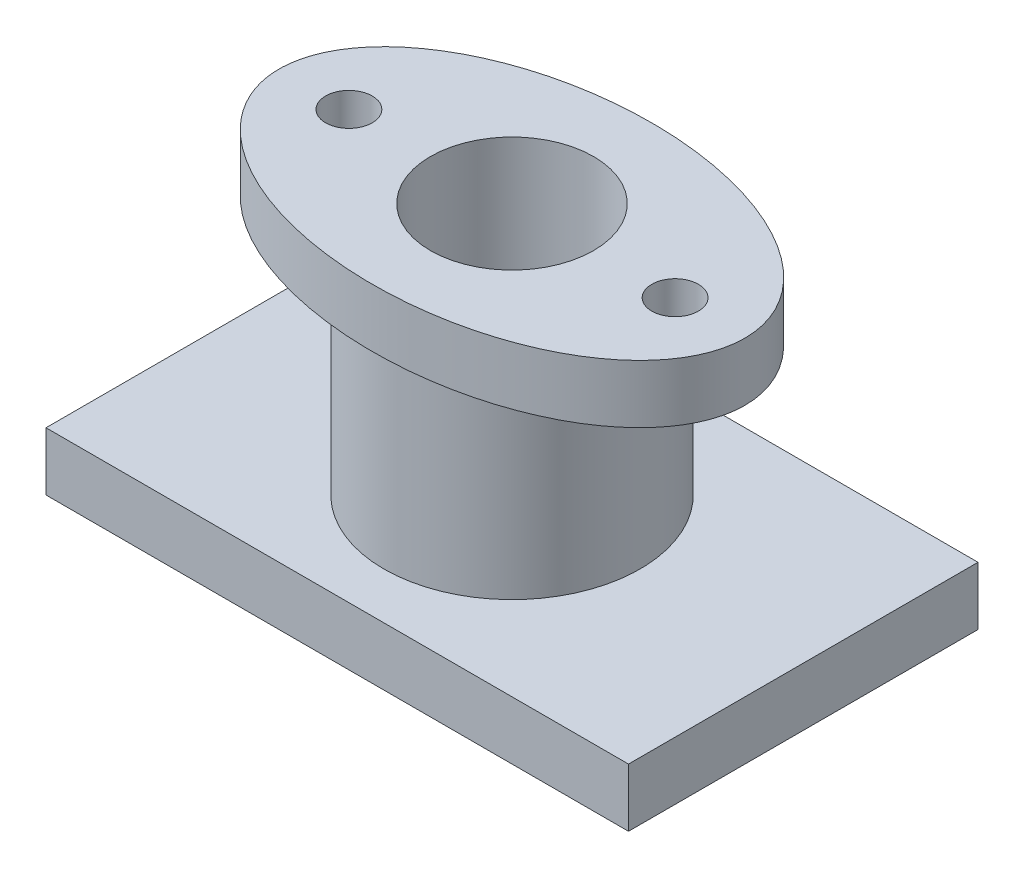
ISO-10303-21;
HEADER;
FILE_DESCRIPTION(('STEP AP214'),'2;1');
FILE_NAME('part.step','',(''),(''),'','','');
FILE_SCHEMA(('AUTOMOTIVE_DESIGN { 1 0 10303 214 1 1 1 1 }'));
ENDSEC;
DATA;
#1=APPLICATION_CONTEXT('core data for automotive mechanical design processes');
#2=APPLICATION_PROTOCOL_DEFINITION('international standard','automotive_design',2000,#1);
#3=PRODUCT_CONTEXT('',#1,'mechanical');
#4=PRODUCT('Part','Part','',(#3));
#5=PRODUCT_RELATED_PRODUCT_CATEGORY('part','',(#4));
#6=PRODUCT_DEFINITION_FORMATION('','',#4);
#7=PRODUCT_DEFINITION_CONTEXT('part definition',#1,'design');
#8=PRODUCT_DEFINITION('design','',#6,#7);
#9=PRODUCT_DEFINITION_SHAPE('','',#8);
#10=(LENGTH_UNIT() NAMED_UNIT(*) SI_UNIT(.MILLI.,.METRE.));
#11=(NAMED_UNIT(*) PLANE_ANGLE_UNIT() SI_UNIT($,.RADIAN.));
#12=(NAMED_UNIT(*) SI_UNIT($,.STERADIAN.) SOLID_ANGLE_UNIT());
#13=UNCERTAINTY_MEASURE_WITH_UNIT(LENGTH_MEASURE(1.E-05),#10,'distance_accuracy_value','');
#14=(GEOMETRIC_REPRESENTATION_CONTEXT(3) GLOBAL_UNCERTAINTY_ASSIGNED_CONTEXT((#13)) GLOBAL_UNIT_ASSIGNED_CONTEXT((#10,
#11,#12)) REPRESENTATION_CONTEXT('',''));
#15=CARTESIAN_POINT('',(0.,0.,0.));
#16=DIRECTION('',(0.,0.,1.));
#17=DIRECTION('',(1.,0.,0.));
#18=AXIS2_PLACEMENT_3D('',#15,#16,#17);
#19=CARTESIAN_POINT('',(75.,15.,45.));
#20=DIRECTION('',(-1.,0.,0.));
#21=DIRECTION('',(0.,0.,1.));
#22=AXIS2_PLACEMENT_3D('',#19,#20,#21);
#23=PLANE('',#22);
#24=DIRECTION('',(0.,0.,-1.));
#25=VECTOR('',#24,1.);
#26=CARTESIAN_POINT('',(75.,0.,45.));
#27=LINE('',#26,#25);
#28=CARTESIAN_POINT('',(75.,0.,45.));
#29=VERTEX_POINT('',#28);
#30=CARTESIAN_POINT('',(75.,0.,-45.));
#31=VERTEX_POINT('',#30);
#32=EDGE_CURVE('E102',#29,#31,#27,.T.);
#33=ORIENTED_EDGE('',*,*,#32,.T.);
#34=DIRECTION('',(0.,-1.,0.));
#35=VECTOR('',#34,1.);
#36=CARTESIAN_POINT('',(75.,15.,-45.));
#37=LINE('',#36,#35);
#38=CARTESIAN_POINT('',(75.,15.,-45.));
#39=VERTEX_POINT('',#38);
#40=EDGE_CURVE('E50',#39,#31,#37,.T.);
#41=ORIENTED_EDGE('',*,*,#40,.F.);
#42=DIRECTION('',(0.,0.,-1.));
#43=VECTOR('',#42,1.);
#44=CARTESIAN_POINT('',(75.,15.,45.));
#45=LINE('',#44,#43);
#46=CARTESIAN_POINT('',(75.,15.,45.));
#47=VERTEX_POINT('',#46);
#48=EDGE_CURVE('E91',#47,#39,#45,.T.);
#49=ORIENTED_EDGE('',*,*,#48,.F.);
#50=DIRECTION('',(0.,-1.,0.));
#51=VECTOR('',#50,1.);
#52=CARTESIAN_POINT('',(75.,15.,45.));
#53=LINE('',#52,#51);
#54=EDGE_CURVE('E103',#47,#29,#53,.T.);
#55=ORIENTED_EDGE('',*,*,#54,.T.);
#56=EDGE_LOOP('',(#33,#41,#49,#55));
#57=FACE_BOUND('',#56,.T.);
#58=ADVANCED_FACE('F39',(#57),#23,.F.);
#59=CARTESIAN_POINT('',(-75.,15.,-45.));
#60=DIRECTION('',(0.,0.,1.));
#61=DIRECTION('',(1.,0.,0.));
#62=AXIS2_PLACEMENT_3D('',#59,#60,#61);
#63=PLANE('',#62);
#64=DIRECTION('',(-1.,0.,0.));
#65=VECTOR('',#64,1.);
#66=CARTESIAN_POINT('',(-75.,0.,-45.));
#67=LINE('',#66,#65);
#68=CARTESIAN_POINT('',(-75.,0.,-45.));
#69=VERTEX_POINT('',#68);
#70=EDGE_CURVE('E98',#31,#69,#67,.T.);
#71=ORIENTED_EDGE('',*,*,#70,.T.);
#72=DIRECTION('',(0.,-1.,0.));
#73=VECTOR('',#72,1.);
#74=CARTESIAN_POINT('',(-75.,15.,-45.));
#75=LINE('',#74,#73);
#76=CARTESIAN_POINT('',(-75.,15.,-45.));
#77=VERTEX_POINT('',#76);
#78=EDGE_CURVE('E93',#77,#69,#75,.T.);
#79=ORIENTED_EDGE('',*,*,#78,.F.);
#80=DIRECTION('',(-1.,0.,0.));
#81=VECTOR('',#80,1.);
#82=CARTESIAN_POINT('',(-75.,15.,-45.));
#83=LINE('',#82,#81);
#84=EDGE_CURVE('E86',#39,#77,#83,.T.);
#85=ORIENTED_EDGE('',*,*,#84,.F.);
#86=ORIENTED_EDGE('',*,*,#40,.T.);
#87=EDGE_LOOP('',(#71,#79,#85,#86));
#88=FACE_BOUND('',#87,.T.);
#89=ADVANCED_FACE('F94',(#88),#63,.F.);
#90=CARTESIAN_POINT('',(-75.,15.,45.));
#91=DIRECTION('',(1.,0.,0.));
#92=DIRECTION('',(0.,0.,-1.));
#93=AXIS2_PLACEMENT_3D('',#90,#91,#92);
#94=PLANE('',#93);
#95=DIRECTION('',(0.,0.,1.));
#96=VECTOR('',#95,1.);
#97=CARTESIAN_POINT('',(-75.,0.,45.));
#98=LINE('',#97,#96);
#99=CARTESIAN_POINT('',(-75.,0.,45.));
#100=VERTEX_POINT('',#99);
#101=EDGE_CURVE('E75',#69,#100,#98,.T.);
#102=ORIENTED_EDGE('',*,*,#101,.T.);
#103=DIRECTION('',(0.,-1.,0.));
#104=VECTOR('',#103,1.);
#105=CARTESIAN_POINT('',(-75.,15.,45.));
#106=LINE('',#105,#104);
#107=CARTESIAN_POINT('',(-75.,15.,45.));
#108=VERTEX_POINT('',#107);
#109=EDGE_CURVE('E97',#108,#100,#106,.T.);
#110=ORIENTED_EDGE('',*,*,#109,.F.);
#111=DIRECTION('',(0.,0.,1.));
#112=VECTOR('',#111,1.);
#113=CARTESIAN_POINT('',(-75.,15.,45.));
#114=LINE('',#113,#112);
#115=EDGE_CURVE('E88',#77,#108,#114,.T.);
#116=ORIENTED_EDGE('',*,*,#115,.F.);
#117=ORIENTED_EDGE('',*,*,#78,.T.);
#118=EDGE_LOOP('',(#102,#110,#116,#117));
#119=FACE_BOUND('',#118,.T.);
#120=ADVANCED_FACE('F100',(#119),#94,.F.);
#121=CARTESIAN_POINT('',(-75.,15.,45.));
#122=DIRECTION('',(0.,0.,-1.));
#123=DIRECTION('',(-1.,0.,0.));
#124=AXIS2_PLACEMENT_3D('',#121,#122,#123);
#125=PLANE('',#124);
#126=DIRECTION('',(1.,0.,0.));
#127=VECTOR('',#126,1.);
#128=CARTESIAN_POINT('',(-75.,0.,45.));
#129=LINE('',#128,#127);
#130=EDGE_CURVE('E76',#100,#29,#129,.T.);
#131=ORIENTED_EDGE('',*,*,#130,.T.);
#132=ORIENTED_EDGE('',*,*,#54,.F.);
#133=DIRECTION('',(1.,0.,0.));
#134=VECTOR('',#133,1.);
#135=CARTESIAN_POINT('',(-75.,15.,45.));
#136=LINE('',#135,#134);
#137=EDGE_CURVE('E54',#108,#47,#136,.T.);
#138=ORIENTED_EDGE('',*,*,#137,.F.);
#139=ORIENTED_EDGE('',*,*,#109,.T.);
#140=EDGE_LOOP('',(#131,#132,#138,#139));
#141=FACE_BOUND('',#140,.T.);
#142=ADVANCED_FACE('F128',(#141),#125,.F.);
#143=CARTESIAN_POINT('',(0.,15.,0.));
#144=DIRECTION('',(0.,-1.,0.));
#145=DIRECTION('',(0.,0.,-1.));
#146=AXIS2_PLACEMENT_3D('',#143,#144,#145);
#147=PLANE('',#146);
#148=CARTESIAN_POINT('',(0.,15.,0.));
#149=DIRECTION('',(0.,-1.,0.));
#150=DIRECTION('',(0.,0.,-1.));
#151=AXIS2_PLACEMENT_3D('',#148,#149,#150);
#152=CIRCLE('',#151,33.);
#153=CARTESIAN_POINT('',(0.,15.,-33.));
#154=VERTEX_POINT('',#153);
#155=EDGE_CURVE('E11',#154,#154,#152,.F.);
#156=ORIENTED_EDGE('',*,*,#155,.F.);
#157=EDGE_LOOP('',(#156));
#158=FACE_BOUND('',#157,.T.);
#159=ORIENTED_EDGE('',*,*,#48,.T.);
#160=ORIENTED_EDGE('',*,*,#84,.T.);
#161=ORIENTED_EDGE('',*,*,#115,.T.);
#162=ORIENTED_EDGE('',*,*,#137,.T.);
#163=EDGE_LOOP('',(#159,#160,#161,#162));
#164=FACE_BOUND('',#163,.T.);
#165=ADVANCED_FACE('F90',(#158,#164),#147,.F.);
#166=CARTESIAN_POINT('',(0.,0.,0.));
#167=DIRECTION('',(0.,-1.,0.));
#168=DIRECTION('',(0.,0.,-1.));
#169=AXIS2_PLACEMENT_3D('',#166,#167,#168);
#170=PLANE('',#169);
#171=CARTESIAN_POINT('',(0.,0.,0.));
#172=DIRECTION('',(0.,1.,0.));
#173=DIRECTION('',(0.,0.,1.));
#174=AXIS2_PLACEMENT_3D('',#171,#172,#173);
#175=CIRCLE('',#174,16.5);
#176=CARTESIAN_POINT('',(0.,0.,16.5));
#177=VERTEX_POINT('',#176);
#178=EDGE_CURVE('E255',#177,#177,#175,.T.);
#179=ORIENTED_EDGE('',*,*,#178,.T.);
#180=EDGE_LOOP('',(#179));
#181=FACE_BOUND('',#180,.T.);
#182=ORIENTED_EDGE('',*,*,#32,.F.);
#183=ORIENTED_EDGE('',*,*,#130,.F.);
#184=ORIENTED_EDGE('',*,*,#101,.F.);
#185=ORIENTED_EDGE('',*,*,#70,.F.);
#186=EDGE_LOOP('',(#182,#183,#184,#185));
#187=FACE_BOUND('',#186,.T.);
#188=ADVANCED_FACE('F116',(#181,#187),#170,.T.);
#189=CARTESIAN_POINT('',(0.,65.,0.));
#190=DIRECTION('',(0.,-1.,0.));
#191=DIRECTION('',(0.,0.,-1.));
#192=AXIS2_PLACEMENT_3D('',#189,#190,#191);
#193=CYLINDRICAL_SURFACE('',#192,33.);
#194=CARTESIAN_POINT('',(0.,65.,0.));
#195=DIRECTION('',(0.,1.,0.));
#196=DIRECTION('',(0.,0.,1.));
#197=AXIS2_PLACEMENT_3D('',#194,#195,#196);
#198=CIRCLE('',#197,33.);
#199=CARTESIAN_POINT('',(0.,65.,33.));
#200=VERTEX_POINT('',#199);
#201=EDGE_CURVE('E108',#200,#200,#198,.T.);
#202=ORIENTED_EDGE('',*,*,#201,.F.);
#203=EDGE_LOOP('',(#202));
#204=FACE_BOUND('',#203,.T.);
#205=ORIENTED_EDGE('',*,*,#155,.T.);
#206=EDGE_LOOP('',(#205));
#207=FACE_BOUND('',#206,.T.);
#208=ADVANCED_FACE('F117',(#204,#207),#193,.T.);
#209=CARTESIAN_POINT('',(0.,80.,0.));
#210=DIRECTION('',(0.,1.,0.));
#211=DIRECTION('',(0.,0.,1.));
#212=AXIS2_PLACEMENT_3D('',#209,#210,#211);
#213=PLANE('',#212);
#214=CARTESIAN_POINT('',(-41.9958461212827,80.,0.));
#215=DIRECTION('',(0.,1.,0.));
#216=DIRECTION('',(0.,0.,1.));
#217=AXIS2_PLACEMENT_3D('',#214,#215,#216);
#218=CIRCLE('',#217,6.);
#219=CARTESIAN_POINT('',(-41.9958461212827,80.,6.));
#220=VERTEX_POINT('',#219);
#221=EDGE_CURVE('E264',#220,#220,#218,.T.);
#222=ORIENTED_EDGE('',*,*,#221,.F.);
#223=EDGE_LOOP('',(#222));
#224=FACE_BOUND('',#223,.T.);
#225=CARTESIAN_POINT('',(41.9958461212827,80.,0.));
#226=DIRECTION('',(0.,1.,0.));
#227=DIRECTION('',(0.,0.,-1.));
#228=AXIS2_PLACEMENT_3D('',#225,#226,#227);
#229=CIRCLE('',#228,6.);
#230=CARTESIAN_POINT('',(41.9958461212827,80.,-6.));
#231=VERTEX_POINT('',#230);
#232=EDGE_CURVE('E256',#231,#231,#229,.T.);
#233=ORIENTED_EDGE('',*,*,#232,.F.);
#234=EDGE_LOOP('',(#233));
#235=FACE_BOUND('',#234,.T.);
#236=CARTESIAN_POINT('',(0.,80.,0.));
#237=DIRECTION('',(0.,1.,0.));
#238=DIRECTION('',(1.,0.,0.));
#239=AXIS2_PLACEMENT_3D('',#236,#237,#238);
#240=ELLIPSE('',#239,60.,36.);
#241=CARTESIAN_POINT('',(60.,80.,0.));
#242=VERTEX_POINT('',#241);
#243=EDGE_CURVE('E224',#242,#242,#240,.T.);
#244=ORIENTED_EDGE('',*,*,#243,.T.);
#245=EDGE_LOOP('',(#244));
#246=FACE_BOUND('',#245,.T.);
#247=CARTESIAN_POINT('',(0.,80.,0.));
#248=DIRECTION('',(0.,1.,0.));
#249=DIRECTION('',(0.,0.,1.));
#250=AXIS2_PLACEMENT_3D('',#247,#248,#249);
#251=CIRCLE('',#250,21.);
#252=CARTESIAN_POINT('',(0.,80.,21.));
#253=VERTEX_POINT('',#252);
#254=EDGE_CURVE('E235',#253,#253,#251,.T.);
#255=ORIENTED_EDGE('',*,*,#254,.F.);
#256=EDGE_LOOP('',(#255));
#257=FACE_BOUND('',#256,.T.);
#258=ADVANCED_FACE('F127',(#224,#235,#246,#257),#213,.T.);
#259=CARTESIAN_POINT('',(0.,65.,0.));
#260=DIRECTION('',(0.,1.,0.));
#261=DIRECTION('',(0.,0.,1.));
#262=AXIS2_PLACEMENT_3D('',#259,#260,#261);
#263=PLANE('',#262);
#264=CARTESIAN_POINT('',(-41.9958461212827,65.,0.));
#265=DIRECTION('',(0.,1.,0.));
#266=DIRECTION('',(0.,0.,1.));
#267=AXIS2_PLACEMENT_3D('',#264,#265,#266);
#268=CIRCLE('',#267,6.);
#269=CARTESIAN_POINT('',(-41.9958461212827,65.,6.));
#270=VERTEX_POINT('',#269);
#271=EDGE_CURVE('E260',#270,#270,#268,.T.);
#272=ORIENTED_EDGE('',*,*,#271,.T.);
#273=EDGE_LOOP('',(#272));
#274=FACE_BOUND('',#273,.T.);
#275=CARTESIAN_POINT('',(41.9958461212827,65.,0.));
#276=DIRECTION('',(0.,1.,0.));
#277=DIRECTION('',(0.,0.,-1.));
#278=AXIS2_PLACEMENT_3D('',#275,#276,#277);
#279=CIRCLE('',#278,6.);
#280=CARTESIAN_POINT('',(41.9958461212827,65.,-6.));
#281=VERTEX_POINT('',#280);
#282=EDGE_CURVE('E265',#281,#281,#279,.T.);
#283=ORIENTED_EDGE('',*,*,#282,.T.);
#284=EDGE_LOOP('',(#283));
#285=FACE_BOUND('',#284,.T.);
#286=ORIENTED_EDGE('',*,*,#201,.T.);
#287=EDGE_LOOP('',(#286));
#288=FACE_BOUND('',#287,.T.);
#289=CARTESIAN_POINT('',(0.,65.,0.));
#290=DIRECTION('',(0.,1.,0.));
#291=DIRECTION('',(1.,0.,0.));
#292=AXIS2_PLACEMENT_3D('',#289,#290,#291);
#293=ELLIPSE('',#292,60.,36.);
#294=CARTESIAN_POINT('',(60.,65.,0.));
#295=VERTEX_POINT('',#294);
#296=EDGE_CURVE('E233',#295,#295,#293,.T.);
#297=ORIENTED_EDGE('',*,*,#296,.F.);
#298=EDGE_LOOP('',(#297));
#299=FACE_BOUND('',#298,.T.);
#300=ADVANCED_FACE('F166',(#274,#285,#288,#299),#263,.F.);
#301=DIRECTION('',(0.,-1.,0.));
#302=VECTOR('',#301,1.);
#303=SURFACE_OF_LINEAR_EXTRUSION('',#240,#302);
#304=ORIENTED_EDGE('',*,*,#243,.F.);
#305=EDGE_LOOP('',(#304));
#306=FACE_BOUND('',#305,.T.);
#307=ORIENTED_EDGE('',*,*,#296,.T.);
#308=EDGE_LOOP('',(#307));
#309=FACE_BOUND('',#308,.T.);
#310=ADVANCED_FACE('F164',(#306,#309),#303,.F.);
#311=CARTESIAN_POINT('',(0.,15.,0.));
#312=DIRECTION('',(0.,1.,0.));
#313=DIRECTION('',(0.,0.,1.));
#314=AXIS2_PLACEMENT_3D('',#311,#312,#313);
#315=CIRCLE('',#314,16.5);
#316=CARTESIAN_POINT('',(0.,15.,16.5));
#317=VERTEX_POINT('',#316);
#318=EDGE_CURVE('E254',#317,#317,#315,.T.);
#319=ORIENTED_EDGE('',*,*,#318,.F.);
#320=EDGE_LOOP('',(#319));
#321=FACE_BOUND('',#320,.T.);
#322=CARTESIAN_POINT('',(0.,15.,0.));
#323=DIRECTION('',(0.,1.,0.));
#324=DIRECTION('',(0.,0.,1.));
#325=AXIS2_PLACEMENT_3D('',#322,#323,#324);
#326=CIRCLE('',#325,21.);
#327=CARTESIAN_POINT('',(0.,15.,21.));
#328=VERTEX_POINT('',#327);
#329=EDGE_CURVE('E229',#328,#328,#326,.T.);
#330=ORIENTED_EDGE('',*,*,#329,.T.);
#331=EDGE_LOOP('',(#330));
#332=FACE_BOUND('',#331,.T.);
#333=ADVANCED_FACE('F132',(#321,#332),#147,.F.);
#334=CARTESIAN_POINT('',(0.,65.,0.));
#335=DIRECTION('',(0.,-1.,0.));
#336=DIRECTION('',(0.,0.,-1.));
#337=AXIS2_PLACEMENT_3D('',#334,#335,#336);
#338=CYLINDRICAL_SURFACE('',#337,21.);
#339=ORIENTED_EDGE('',*,*,#329,.F.);
#340=EDGE_LOOP('',(#339));
#341=FACE_BOUND('',#340,.T.);
#342=ORIENTED_EDGE('',*,*,#254,.T.);
#343=EDGE_LOOP('',(#342));
#344=FACE_BOUND('',#343,.T.);
#345=ADVANCED_FACE('F176',(#341,#344),#338,.F.);
#346=CARTESIAN_POINT('',(0.,0.,0.));
#347=DIRECTION('',(0.,1.,0.));
#348=DIRECTION('',(0.,0.,1.));
#349=AXIS2_PLACEMENT_3D('',#346,#347,#348);
#350=CYLINDRICAL_SURFACE('',#349,16.5);
#351=ORIENTED_EDGE('',*,*,#178,.F.);
#352=EDGE_LOOP('',(#351));
#353=FACE_BOUND('',#352,.T.);
#354=ORIENTED_EDGE('',*,*,#318,.T.);
#355=EDGE_LOOP('',(#354));
#356=FACE_BOUND('',#355,.T.);
#357=ADVANCED_FACE('F178',(#353,#356),#350,.F.);
#358=CARTESIAN_POINT('',(41.9958461212827,65.,0.));
#359=DIRECTION('',(0.,1.,0.));
#360=DIRECTION('',(0.,0.,1.));
#361=AXIS2_PLACEMENT_3D('',#358,#359,#360);
#362=CYLINDRICAL_SURFACE('',#361,6.);
#363=ORIENTED_EDGE('',*,*,#282,.F.);
#364=EDGE_LOOP('',(#363));
#365=FACE_BOUND('',#364,.T.);
#366=ORIENTED_EDGE('',*,*,#232,.T.);
#367=EDGE_LOOP('',(#366));
#368=FACE_BOUND('',#367,.T.);
#369=ADVANCED_FACE('F194',(#365,#368),#362,.F.);
#370=CARTESIAN_POINT('',(-41.9958461212827,65.,0.));
#371=DIRECTION('',(0.,1.,0.));
#372=DIRECTION('',(0.,0.,1.));
#373=AXIS2_PLACEMENT_3D('',#370,#371,#372);
#374=CYLINDRICAL_SURFACE('',#373,6.);
#375=ORIENTED_EDGE('',*,*,#271,.F.);
#376=EDGE_LOOP('',(#375));
#377=FACE_BOUND('',#376,.T.);
#378=ORIENTED_EDGE('',*,*,#221,.T.);
#379=EDGE_LOOP('',(#378));
#380=FACE_BOUND('',#379,.T.);
#381=ADVANCED_FACE('F203',(#377,#380),#374,.F.);
#382=CLOSED_SHELL('',(#58,#89,#120,#142,#165,#188,#208,#258,#300,#310,#333,#345,#357,#369,#381));
#383=MANIFOLD_SOLID_BREP('B2',#382);
#384=ADVANCED_BREP_SHAPE_REPRESENTATION('',(#18,#383),#14);
#385=SHAPE_DEFINITION_REPRESENTATION(#9,#384);
ENDSEC;
END-ISO-10303-21;
